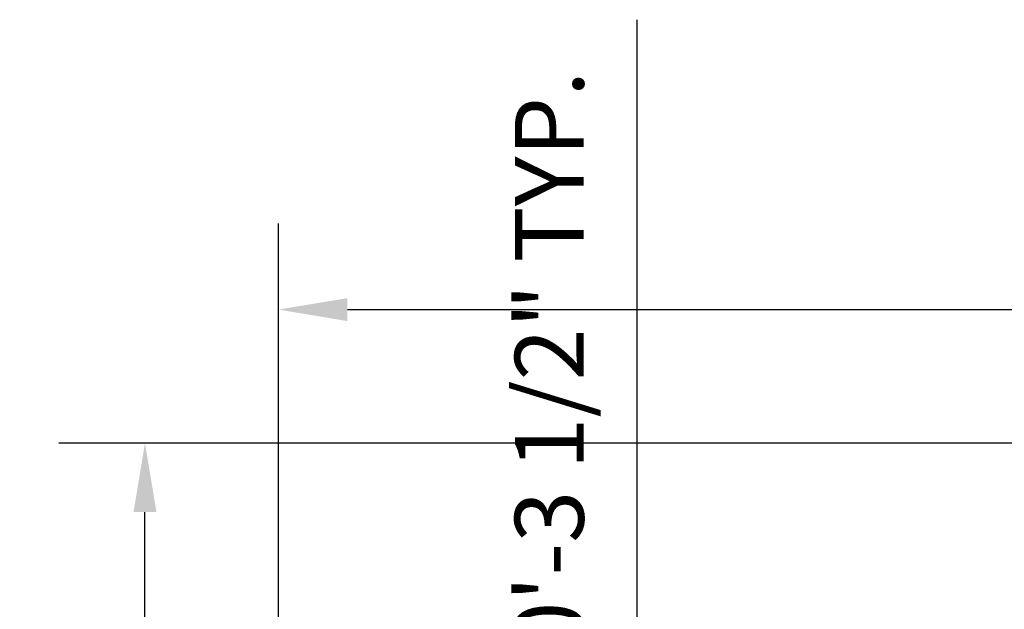
# Model space of a CAD drawing. Units: millimetres. Extents: x 7894 to 8038, y 6851 to 6951.
# Tile 46 of 49: x 7936.33 to 7950.62, y 6942.2 to 6950.75. Entities that reach past the tile are written whole.
import ezdxf

# ---------------------------------------------------------------- set-up
doc = ezdxf.new("R2010")
doc.units = ezdxf.units.MM
doc.layers.add('A-ANNO-DIMS', color=2, linetype='Continuous', lineweight=18)
doc.styles.get("Standard").update_dxf_attribs({"font": 'arial.ttf'})
doc.dimstyles.new('ISO-25', dxfattribs={"dimtxt": 1, "dimasz": 1, "dimexe": 1.25, "dimexo": 0.625, "dimtad": 1, "dimdec": 0, "dimlunit": 4, "dimtxsty": 'Standard', "dimcen": 2.5, "dimclrt": 1, "dimadec": 0, "dimazin": 0, "dimtfac": 1, "dimtdec": 0, "dimtmove": 0, "dimatfit": 3, "dimfxl": 1, "dimarcsym": 0})

# ---------------------------------------------------------------- blocks, each defined once
blk = doc.blocks.new('*D17')
at = {"layer": 'A-ANNO-DIMS', "color": 0, "lineweight": -2, "transparency": 16777216}
for p, q in [((7945.291, 6935.394), (7945.291, 6950.748)), ((7945.192, 6935.394), (7944.041, 6935.394)), ((7945.291, 6932.885), (7945.291, 6934.394)), ((7945.192, 6931.885), (7944.041, 6931.885))]:
    blk.add_line(p, q, dxfattribs=at)
at = {"layer": 'A-ANNO-DIMS', "color": 0, "transparency": 16777216}
for points in [[(7945.124, 6934.394), (7945.457, 6934.394), (7945.291, 6935.394)], [(7945.124, 6932.885), (7945.457, 6932.885), (7945.291, 6931.885)]]:
    blk.add_solid(points, dxfattribs=at)
at = {"layer": 'Defpoints', "color": 0, "transparency": 16777216}
for p in [(7945.291, 6935.394), (7945.817, 6935.394), (7945.817, 6931.885)]:
    blk.add_point(p, dxfattribs=at)
at = {"layer": 'A-ANNO-DIMS', "color": 1, "transparency": 16777216, "insert": (7944.148, 6943.571), "char_height": 1, "attachment_point": 5, "rotation": 90}
blk.add_mtext('FINIAL 0\'-3 1/2" TYP.', dxfattribs=at)
blk = doc.blocks.new('*D23')
at = {"layer": 'A-ANNO-DIMS', "color": 0, "lineweight": -2, "transparency": 16777216}
for p, q in [((7940.089, 6907.098), (7940.089, 6947.793)), ((7971.936, 6928.989), (7971.936, 6947.793)), ((7941.089, 6946.543), (7970.936, 6946.543))]:
    blk.add_line(p, q, dxfattribs=at)
at = {"layer": 'A-ANNO-DIMS', "color": 0, "transparency": 16777216}
for points in [[(7941.089, 6946.709), (7941.089, 6946.376), (7940.089, 6946.543)], [(7970.936, 6946.709), (7970.936, 6946.376), (7971.936, 6946.543)]]:
    blk.add_solid(points, dxfattribs=at)
at = {"layer": 'Defpoints', "color": 0, "transparency": 16777216}
for p in [(7971.936, 6946.543), (7971.936, 6928.364), (7940.089, 6906.473)]:
    blk.add_point(p, dxfattribs=at)
at = {"layer": 'A-ANNO-DIMS', "color": 1, "transparency": 16777216, "insert": (7956.012, 6947.678), "char_height": 1, "attachment_point": 5}
blk.add_mtext('2\'-8"', dxfattribs=at)
blk = doc.blocks.new('*D24')
at = {"layer": 'A-ANNO-DIMS', "color": 0, "lineweight": -2, "transparency": 16777216}
for p, q in [((7953.341, 6944.606), (7936.902, 6944.606)), ((7938.152, 6907.473), (7938.152, 6943.606)), ((7939.464, 6906.473), (7936.902, 6906.473))]:
    blk.add_line(p, q, dxfattribs=at)
at = {"layer": 'A-ANNO-DIMS', "color": 0, "transparency": 16777216}
for points in [[(7937.986, 6943.606), (7938.319, 6943.606), (7938.152, 6944.606)], [(7937.986, 6907.473), (7938.319, 6907.473), (7938.152, 6906.473)]]:
    blk.add_solid(points, dxfattribs=at)
at = {"layer": 'Defpoints', "color": 0, "transparency": 16777216}
for p in [(7938.152, 6944.606), (7953.966, 6944.606), (7940.089, 6906.473)]:
    blk.add_point(p, dxfattribs=at)
at = {"layer": 'A-ANNO-DIMS', "color": 1, "transparency": 16777216, "insert": (7937.016, 6925.539), "char_height": 1, "attachment_point": 5, "rotation": 90}
blk.add_mtext('3\'-2"', dxfattribs=at)

msp = doc.modelspace()

# ---------------------------------------------------------------- dimensions: what is measured, and where the dimension line sits
at = {"layer": 'A-ANNO-DIMS'}
dim = msp.add_linear_dim(base=(7945.291, 6935.394), p1=(7945.817, 6931.885), p2=(7945.817, 6935.394), angle=90, text='FINIAL <> TYP.', dimstyle='ISO-25', override={"dimdec": 1, "dimlfac": 1, "dimrnd": 0, "dimzin": 1, "dimdsep": 46, "dimlunit": 4, "dimfrac": 2}, dxfattribs=at)
dim.commit()
dim.dimension.update_dxf_attribs({"geometry": '*D17', "text_midpoint": (7944.148, 6943.571)})
dim = msp.add_linear_dim(base=(7971.936, 6946.543), p1=(7940.089, 6906.473), p2=(7971.936, 6928.364), dimstyle='ISO-25', override={"dimdec": 1, "dimlfac": 1, "dimrnd": 0, "dimzin": 1, "dimdsep": 46, "dimlunit": 4, "dimfrac": 2}, dxfattribs=at)
dim.commit()
dim.dimension.update_dxf_attribs({"geometry": '*D23', "text_midpoint": (7956.012, 6947.678)})
dim = msp.add_linear_dim(base=(7938.152, 6944.606), p1=(7940.089, 6906.473), p2=(7953.966, 6944.606), angle=90, dimstyle='ISO-25', override={"dimdec": 1, "dimlfac": 1, "dimrnd": 0, "dimzin": 1, "dimdsep": 46, "dimlunit": 4, "dimfrac": 2}, dxfattribs=at)
dim.commit()
dim.dimension.update_dxf_attribs({"geometry": '*D24', "text_midpoint": (7937.016, 6925.539)})

doc.saveas('drawing.dxf')
